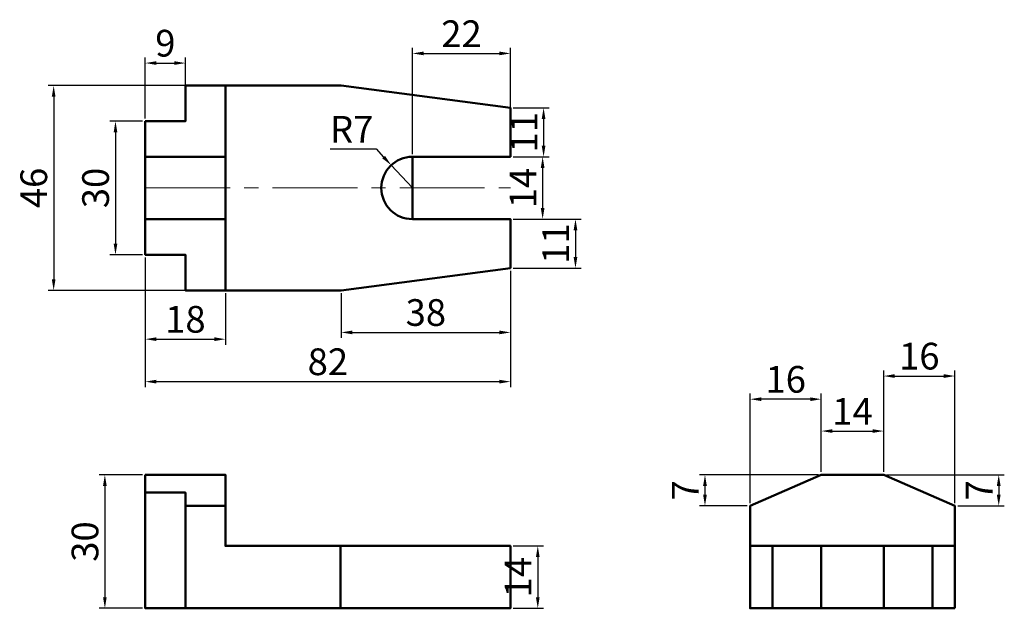
# Model space of a CAD drawing. Units: millimetres. Extents: x 44 to 265, y 73 to 205.
import ezdxf

# ---------------------------------------------------------------- set-up
doc = ezdxf.new("R2010")
doc.units = ezdxf.units.MM
doc.linetypes.add('CENTER2', pattern=[28.575, 19.05, -3.175, 3.175, -3.175])
for name, color, linetype, lineweight in [('M-CNTR', 1, 'CENTER2', 18), ('M-DIMS', 2, 'Continuous', 25), ('M-OUTL', 7, 'Continuous', 50)]:
    doc.layers.add(name, color=color, linetype=linetype, lineweight=lineweight)
doc.styles.get("Standard").update_dxf_attribs({"font": 'arial.ttf'})
doc.dimstyles.new('ISO-25', dxfattribs={"dimtxt": 6, "dimasz": 2.5, "dimexe": 1.25, "dimexo": 0.625, "dimtad": 1, "dimtoh": 1, "dimdec": 0, "dimtxsty": 'Standard', "dimcen": 2.5, "dimadec": 0, "dimazin": 0, "dimtfac": 1, "dimtdec": 0, "dimtmove": 0, "dimatfit": 3, "dimfxl": 1, "dimarcsym": 0})

# ---------------------------------------------------------------- blocks, each defined once
blk = doc.blocks.new('*D1')
at = {"layer": 'Defpoints', "color": 0, "transparency": 16777216}
for p in [(72.34, 152.49), (90.34, 144.49), (90.34, 133.53)]:
    blk.add_point(p, dxfattribs=at)
at = {"layer": 'M-DIMS', "color": 0, "lineweight": -2, "transparency": 16777216}
for p, q in [((72.34, 151.86), (72.34, 132.28)), ((90.34, 143.86), (90.34, 132.28)), ((74.84, 133.53), (87.84, 133.53))]:
    blk.add_line(p, q, dxfattribs=at)
at = {"layer": 'M-DIMS', "color": 0, "transparency": 16777216}
for points in [[(74.84, 133.95), (74.84, 133.11), (72.34, 133.53)], [(87.84, 133.95), (87.84, 133.11), (90.34, 133.53)]]:
    blk.add_solid(points, dxfattribs=at)
at = {"layer": 'M-DIMS', "color": 0, "transparency": 16777216, "insert": (81.34, 137.22), "char_height": 6, "attachment_point": 5}
blk.add_mtext('18', dxfattribs=at)
blk = doc.blocks.new('*D2')
at = {"layer": 'Defpoints', "color": 0, "transparency": 16777216}
for p in [(90.34, 190.49), (51.76, 144.49), (90.34, 144.49)]:
    blk.add_point(p, dxfattribs=at)
at = {"layer": 'M-DIMS', "color": 0, "lineweight": -2, "transparency": 16777216}
for p, q in [((89.71, 190.49), (50.51, 190.49)), ((51.76, 187.99), (51.76, 146.99)), ((89.71, 144.49), (50.51, 144.49))]:
    blk.add_line(p, q, dxfattribs=at)
at = {"layer": 'M-DIMS', "color": 0, "transparency": 16777216}
for points in [[(51.34, 187.99), (52.17, 187.99), (51.76, 190.49)], [(51.34, 146.99), (52.17, 146.99), (51.76, 144.49)]]:
    blk.add_solid(points, dxfattribs=at)
at = {"layer": 'M-DIMS', "color": 0, "transparency": 16777216, "insert": (48.07, 167.49), "char_height": 6, "attachment_point": 5, "rotation": 90}
blk.add_mtext('46', dxfattribs=at)
blk = doc.blocks.new('*D3')
at = {"layer": 'Defpoints', "color": 0, "transparency": 16777216}
for p in [(72.34, 182.49), (65.64, 152.49), (72.34, 152.49)]:
    blk.add_point(p, dxfattribs=at)
at = {"layer": 'M-DIMS', "color": 0, "lineweight": -2, "transparency": 16777216}
for p, q in [((71.71, 182.49), (64.39, 182.49)), ((65.64, 179.99), (65.64, 154.99)), ((71.71, 152.49), (64.39, 152.49))]:
    blk.add_line(p, q, dxfattribs=at)
at = {"layer": 'M-DIMS', "color": 0, "transparency": 16777216}
for points in [[(65.23, 179.99), (66.06, 179.99), (65.64, 182.49)], [(65.23, 154.99), (66.06, 154.99), (65.64, 152.49)]]:
    blk.add_solid(points, dxfattribs=at)
at = {"layer": 'M-DIMS', "color": 0, "transparency": 16777216, "insert": (61.95, 167.49), "char_height": 6, "attachment_point": 5, "rotation": 90}
blk.add_mtext('30', dxfattribs=at)
blk = doc.blocks.new('*D4')
at = {"layer": 'Defpoints', "color": 0, "transparency": 16777216}
for p in [(81.34, 195.54), (72.34, 182.49), (81.34, 182.49)]:
    blk.add_point(p, dxfattribs=at)
at = {"layer": 'M-DIMS', "color": 0, "lineweight": -2, "transparency": 16777216}
for p, q in [((72.34, 183.11), (72.34, 196.79)), ((81.34, 183.11), (81.34, 196.79)), ((74.84, 195.54), (78.84, 195.54))]:
    blk.add_line(p, q, dxfattribs=at)
at = {"layer": 'M-DIMS', "color": 0, "transparency": 16777216}
for points in [[(74.84, 195.96), (74.84, 195.13), (72.34, 195.54)], [(78.84, 195.96), (78.84, 195.13), (81.34, 195.54)]]:
    blk.add_solid(points, dxfattribs=at)
at = {"layer": 'M-DIMS', "color": 0, "transparency": 16777216, "insert": (76.84, 199.23), "char_height": 6, "attachment_point": 5}
blk.add_mtext('9', dxfattribs=at)
blk = doc.blocks.new('*D5')
at = {"layer": 'Defpoints', "color": 0, "transparency": 16777216}
for p in [(154.34, 197.71), (132.34, 174.49), (154.34, 174.49)]:
    blk.add_point(p, dxfattribs=at)
at = {"layer": 'M-DIMS', "color": 0, "lineweight": -2, "transparency": 16777216}
for p, q in [((132.34, 175.11), (132.34, 198.96)), ((134.84, 197.71), (151.84, 197.71)), ((154.34, 175.11), (154.34, 198.96))]:
    blk.add_line(p, q, dxfattribs=at)
at = {"layer": 'M-DIMS', "color": 0, "transparency": 16777216}
for points in [[(134.84, 198.13), (134.84, 197.3), (132.34, 197.71)], [(151.84, 198.13), (151.84, 197.3), (154.34, 197.71)]]:
    blk.add_solid(points, dxfattribs=at)
at = {"layer": 'M-DIMS', "color": 0, "transparency": 16777216, "insert": (143.34, 201.35), "char_height": 6, "attachment_point": 5}
blk.add_mtext('22', dxfattribs=at)
blk = doc.blocks.new('*D6')
at = {"layer": 'Defpoints', "color": 0, "transparency": 16777216}
for p in [(127.56, 172.61), (132.34, 167.49)]:
    blk.add_point(p, dxfattribs=at)
at = {"layer": 'M-DIMS', "color": 0, "lineweight": -2, "transparency": 16777216}
for p, q in [((113.85, 176.26), (124.15, 176.26)), ((124.15, 176.26), (125.86, 174.43)), ((132.34, 167.49), (127.56, 172.61))]:
    blk.add_line(p, q, dxfattribs=at)
at = {"layer": 'M-DIMS', "color": 0, "transparency": 16777216}
blk.add_solid([(126.16, 174.72), (125.55, 174.15), (127.56, 172.61)], dxfattribs=at)
at = {"layer": 'M-DIMS', "color": 0, "transparency": 16777216, "insert": (118.69, 179.89), "char_height": 6, "attachment_point": 5}
blk.add_mtext('R7', dxfattribs=at)
blk = doc.blocks.new('*D7')
at = {"layer": 'Defpoints', "color": 0, "transparency": 16777216}
for p in [(154.34, 185.49), (154.34, 174.49), (161.78, 174.49)]:
    blk.add_point(p, dxfattribs=at)
at = {"layer": 'M-DIMS', "color": 0, "lineweight": -2, "transparency": 16777216}
for p, q in [((154.96, 185.49), (163.03, 185.49)), ((161.78, 182.99), (161.78, 176.99)), ((154.96, 174.49), (163.03, 174.49))]:
    blk.add_line(p, q, dxfattribs=at)
at = {"layer": 'M-DIMS', "color": 0, "transparency": 16777216}
for points in [[(161.36, 182.99), (162.2, 182.99), (161.78, 185.49)], [(161.36, 176.99), (162.2, 176.99), (161.78, 174.49)]]:
    blk.add_solid(points, dxfattribs=at)
at = {"layer": 'M-DIMS', "color": 0, "transparency": 16777216, "insert": (158.14, 179.99), "char_height": 6, "attachment_point": 5, "rotation": 90}
blk.add_mtext('11', dxfattribs=at)
blk = doc.blocks.new('*D8')
at = {"layer": 'Defpoints', "color": 0, "transparency": 16777216}
for p in [(154.34, 174.49), (154.34, 160.49), (161.56, 160.49)]:
    blk.add_point(p, dxfattribs=at)
at = {"layer": 'M-DIMS', "color": 0, "lineweight": -2, "transparency": 16777216}
for p, q in [((154.96, 174.49), (162.81, 174.49)), ((161.56, 171.99), (161.56, 162.99)), ((154.96, 160.49), (162.81, 160.49))]:
    blk.add_line(p, q, dxfattribs=at)
at = {"layer": 'M-DIMS', "color": 0, "transparency": 16777216}
for points in [[(161.15, 171.99), (161.98, 171.99), (161.56, 174.49)], [(161.15, 162.99), (161.98, 162.99), (161.56, 160.49)]]:
    blk.add_solid(points, dxfattribs=at)
at = {"layer": 'M-DIMS', "color": 0, "transparency": 16777216, "insert": (157.93, 167.49), "char_height": 6, "attachment_point": 5, "rotation": 90}
blk.add_mtext('14', dxfattribs=at)
blk = doc.blocks.new('*D9')
at = {"layer": 'Defpoints', "color": 0, "transparency": 16777216}
for p in [(154.34, 160.49), (154.34, 149.49), (168.94, 149.49)]:
    blk.add_point(p, dxfattribs=at)
at = {"layer": 'M-DIMS', "color": 0, "lineweight": -2, "transparency": 16777216}
for p, q in [((154.96, 160.49), (170.19, 160.49)), ((168.94, 157.99), (168.94, 151.99)), ((154.96, 149.49), (170.19, 149.49))]:
    blk.add_line(p, q, dxfattribs=at)
at = {"layer": 'M-DIMS', "color": 0, "transparency": 16777216}
for points in [[(168.52, 157.99), (169.36, 157.99), (168.94, 160.49)], [(168.52, 151.99), (169.36, 151.99), (168.94, 149.49)]]:
    blk.add_solid(points, dxfattribs=at)
at = {"layer": 'M-DIMS', "color": 0, "transparency": 16777216, "insert": (165.3, 154.99), "char_height": 6, "attachment_point": 5, "rotation": 90}
blk.add_mtext('11', dxfattribs=at)
blk = doc.blocks.new('*D10')
at = {"layer": 'Defpoints', "color": 0, "transparency": 16777216}
for p in [(154.34, 149.49), (116.34, 144.49), (154.34, 135.05)]:
    blk.add_point(p, dxfattribs=at)
at = {"layer": 'M-DIMS', "color": 0, "lineweight": -2, "transparency": 16777216}
for p, q in [((154.34, 148.86), (154.34, 133.8)), ((116.34, 143.86), (116.34, 133.8)), ((118.84, 135.05), (151.84, 135.05))]:
    blk.add_line(p, q, dxfattribs=at)
at = {"layer": 'M-DIMS', "color": 0, "transparency": 16777216}
for points in [[(118.84, 135.46), (118.84, 134.63), (116.34, 135.05)], [(151.84, 135.46), (151.84, 134.63), (154.34, 135.05)]]:
    blk.add_solid(points, dxfattribs=at)
at = {"layer": 'M-DIMS', "color": 0, "transparency": 16777216, "insert": (135.34, 138.74), "char_height": 6, "attachment_point": 5}
blk.add_mtext('38', dxfattribs=at)
blk = doc.blocks.new('*D11')
at = {"layer": 'Defpoints', "color": 0, "transparency": 16777216}
for p in [(72.34, 152.49), (154.34, 149.49), (154.34, 123.99)]:
    blk.add_point(p, dxfattribs=at)
at = {"layer": 'M-DIMS', "color": 0, "lineweight": -2, "transparency": 16777216}
for p, q in [((72.34, 151.86), (72.34, 122.74)), ((154.34, 148.86), (154.34, 122.74)), ((74.84, 123.99), (151.84, 123.99))]:
    blk.add_line(p, q, dxfattribs=at)
at = {"layer": 'M-DIMS', "color": 0, "transparency": 16777216}
for points in [[(74.84, 124.41), (74.84, 123.57), (72.34, 123.99)], [(151.84, 124.41), (151.84, 123.57), (154.34, 123.99)]]:
    blk.add_solid(points, dxfattribs=at)
at = {"layer": 'M-DIMS', "color": 0, "transparency": 16777216, "insert": (113.34, 127.68), "char_height": 6, "attachment_point": 5}
blk.add_mtext('82', dxfattribs=at)
blk = doc.blocks.new('*D12')
at = {"layer": 'Defpoints', "color": 0, "transparency": 16777216}
for p in [(72.34, 103.08), (63.26, 73.08), (72.34, 73.08)]:
    blk.add_point(p, dxfattribs=at)
at = {"layer": 'M-DIMS', "color": 0, "lineweight": -2, "transparency": 16777216}
for p, q in [((71.71, 103.08), (62.01, 103.08)), ((63.26, 100.58), (63.26, 75.58)), ((71.71, 73.08), (62.01, 73.08))]:
    blk.add_line(p, q, dxfattribs=at)
at = {"layer": 'M-DIMS', "color": 0, "transparency": 16777216}
for points in [[(62.84, 100.58), (63.67, 100.58), (63.26, 103.08)], [(62.84, 75.58), (63.67, 75.58), (63.26, 73.08)]]:
    blk.add_solid(points, dxfattribs=at)
at = {"layer": 'M-DIMS', "color": 0, "transparency": 16777216, "insert": (59.57, 88.08), "char_height": 6, "attachment_point": 5, "rotation": 90}
blk.add_mtext('30', dxfattribs=at)
blk = doc.blocks.new('*D13')
at = {"layer": 'Defpoints', "color": 0, "transparency": 16777216}
for p in [(154.34, 87.08), (154.34, 73.08), (160.48, 73.08)]:
    blk.add_point(p, dxfattribs=at)
at = {"layer": 'M-DIMS', "color": 0, "lineweight": -2, "transparency": 16777216}
for p, q in [((154.96, 87.08), (161.73, 87.08)), ((160.48, 84.58), (160.48, 75.58)), ((154.96, 73.08), (161.73, 73.08))]:
    blk.add_line(p, q, dxfattribs=at)
at = {"layer": 'M-DIMS', "color": 0, "transparency": 16777216}
for points in [[(160.06, 84.58), (160.89, 84.58), (160.48, 87.08)], [(160.06, 75.58), (160.89, 75.58), (160.48, 73.08)]]:
    blk.add_solid(points, dxfattribs=at)
at = {"layer": 'M-DIMS', "color": 0, "transparency": 16777216, "insert": (156.84, 80.08), "char_height": 6, "attachment_point": 5, "rotation": 90}
blk.add_mtext('14', dxfattribs=at)
blk = doc.blocks.new('*D14')
at = {"layer": 'Defpoints', "color": 0, "transparency": 16777216}
for p in [(224.15, 103.08), (198.02, 96.08), (208.15, 96.08)]:
    blk.add_point(p, dxfattribs=at)
at = {"layer": 'M-DIMS', "color": 0, "lineweight": -2, "transparency": 16777216}
for p, q in [((223.52, 103.08), (196.77, 103.08)), ((198.02, 100.58), (198.02, 98.58)), ((207.52, 96.08), (196.77, 96.08))]:
    blk.add_line(p, q, dxfattribs=at)
at = {"layer": 'M-DIMS', "color": 0, "transparency": 16777216}
for points in [[(197.6, 100.58), (198.44, 100.58), (198.02, 103.08)], [(197.6, 98.58), (198.44, 98.58), (198.02, 96.08)]]:
    blk.add_solid(points, dxfattribs=at)
at = {"layer": 'M-DIMS', "color": 0, "transparency": 16777216, "insert": (194.39, 99.58), "char_height": 6, "attachment_point": 5, "rotation": 90}
blk.add_mtext('7', dxfattribs=at)
blk = doc.blocks.new('*D15')
at = {"layer": 'Defpoints', "color": 0, "transparency": 16777216}
for p in [(238.15, 103.08), (254.15, 96.08), (263.99, 96.08)]:
    blk.add_point(p, dxfattribs=at)
at = {"layer": 'M-DIMS', "color": 0, "lineweight": -2, "transparency": 16777216}
for p, q in [((238.77, 103.08), (265.24, 103.08)), ((263.99, 100.58), (263.99, 98.58)), ((254.77, 96.08), (265.24, 96.08))]:
    blk.add_line(p, q, dxfattribs=at)
at = {"layer": 'M-DIMS', "color": 0, "transparency": 16777216}
for points in [[(263.57, 100.58), (264.41, 100.58), (263.99, 103.08)], [(263.57, 98.58), (264.41, 98.58), (263.99, 96.08)]]:
    blk.add_solid(points, dxfattribs=at)
at = {"layer": 'M-DIMS', "color": 0, "transparency": 16777216, "insert": (260.37, 99.58), "char_height": 6, "attachment_point": 5, "rotation": 90}
blk.add_mtext('7', dxfattribs=at)
blk = doc.blocks.new('*D16')
at = {"layer": 'Defpoints', "color": 0, "transparency": 16777216}
for p in [(208.15, 120.05), (224.15, 103.08), (208.15, 96.08)]:
    blk.add_point(p, dxfattribs=at)
at = {"layer": 'M-DIMS', "color": 0, "lineweight": -2, "transparency": 16777216}
for p, q in [((208.15, 96.71), (208.15, 121.3)), ((221.65, 120.05), (210.65, 120.05)), ((224.15, 103.71), (224.15, 121.3))]:
    blk.add_line(p, q, dxfattribs=at)
at = {"layer": 'M-DIMS', "color": 0, "transparency": 16777216}
for points in [[(210.65, 120.46), (210.65, 119.63), (208.15, 120.05)], [(221.65, 120.46), (221.65, 119.63), (224.15, 120.05)]]:
    blk.add_solid(points, dxfattribs=at)
at = {"layer": 'M-DIMS', "color": 0, "transparency": 16777216, "insert": (216.15, 123.73), "char_height": 6, "attachment_point": 5}
blk.add_mtext('16', dxfattribs=at)
blk = doc.blocks.new('*D17')
at = {"layer": 'Defpoints', "color": 0, "transparency": 16777216}
for p in [(238.15, 112.89), (224.15, 103.08), (238.15, 103.08)]:
    blk.add_point(p, dxfattribs=at)
at = {"layer": 'M-DIMS', "color": 0, "lineweight": -2, "transparency": 16777216}
for p, q in [((224.15, 103.71), (224.15, 114.14)), ((226.65, 112.89), (235.65, 112.89)), ((238.15, 103.71), (238.15, 114.14))]:
    blk.add_line(p, q, dxfattribs=at)
at = {"layer": 'M-DIMS', "color": 0, "transparency": 16777216}
for points in [[(226.65, 113.31), (226.65, 112.47), (224.15, 112.89)], [(235.65, 113.31), (235.65, 112.47), (238.15, 112.89)]]:
    blk.add_solid(points, dxfattribs=at)
at = {"layer": 'M-DIMS', "color": 0, "transparency": 16777216, "insert": (231.15, 116.53), "char_height": 6, "attachment_point": 5}
blk.add_mtext('14', dxfattribs=at)
blk = doc.blocks.new('*D18')
at = {"layer": 'Defpoints', "color": 0, "transparency": 16777216}
for p in [(254.15, 125.25), (238.15, 103.08), (254.15, 96.08)]:
    blk.add_point(p, dxfattribs=at)
at = {"layer": 'M-DIMS', "color": 0, "lineweight": -2, "transparency": 16777216}
for p, q in [((238.15, 103.71), (238.15, 126.5)), ((254.15, 96.71), (254.15, 126.5)), ((240.65, 125.25), (251.65, 125.25))]:
    blk.add_line(p, q, dxfattribs=at)
at = {"layer": 'M-DIMS', "color": 0, "transparency": 16777216}
for points in [[(240.65, 125.67), (240.65, 124.83), (238.15, 125.25)], [(251.65, 125.67), (251.65, 124.83), (254.15, 125.25)]]:
    blk.add_solid(points, dxfattribs=at)
at = {"layer": 'M-DIMS', "color": 0, "transparency": 16777216, "insert": (246.15, 128.94), "char_height": 6, "attachment_point": 5}
blk.add_mtext('16', dxfattribs=at)

msp = doc.modelspace()

# ---------------------------------------------------------------- linework, layer by layer
at = {"layer": 'M-CNTR'}
msp.add_line((72.34, 167.49), (154.34, 167.49), dxfattribs=at)
at = {"layer": 'M-OUTL'}
for p, q in [((90.34, 190.49), (90.34, 144.49)), ((90.34, 174.49), (72.34, 174.49)), ((90.34, 160.49), (72.34, 160.49)), ((90.34, 96.08), (81.34, 96.08)), ((116.14, 87.08), (116.14, 73.08)), ((208.15, 87.08), (254.15, 87.08)), ((213.15, 73.08), (213.15, 87.08)), ((224.15, 73.08), (224.15, 87.08)), ((238.15, 73.08), (238.15, 87.08)), ((249.15, 73.08), (249.15, 87.08))]:
    msp.add_line(p, q, dxfattribs=at)
for points in [[(72.34, 182.49), (81.34, 182.49), (81.34, 190.49), (90.34, 190.49), (116.34, 190.49), (154.34, 185.49), (154.34, 174.49), (132.34, 174.49)], [(72.34, 99.08), (81.34, 99.08), (81.34, 73.08)]]:
    msp.add_lwpolyline(points, dxfattribs=at)
msp.add_lwpolyline([(72.34, 182.49), (72.34, 152.49), (81.34, 152.49), (81.34, 144.49), (90.34, 144.49), (116.34, 144.49), (154.34, 149.49), (154.34, 160.49), (132.34, 160.49, -1), (132.34, 174.49), (132.34, 160.49)], format="xyb", dxfattribs=at)
for points in [[(72.34, 103.08), (90.34, 103.08), (90.34, 87.08), (154.34, 87.08), (154.34, 73.08), (72.34, 73.08)], [(254.15, 73.08), (254.15, 96.08), (238.15, 103.08), (224.15, 103.08), (208.15, 96.08), (208.15, 73.08)]]:
    msp.add_lwpolyline(points, close=True, dxfattribs=at)

# ---------------------------------------------------------------- dimensions: what is measured, and where the dimension line sits
at = {"layer": 'M-DIMS'}
for base, p1, p2, picture, middle in [((154.34, 197.71), (132.34, 174.49), (154.34, 174.49), '*D5', (143.34, 201.35)), ((81.34, 195.54), (72.34, 182.49), (81.34, 182.49), '*D4', (76.84, 199.23)), ((90.34, 133.53), (72.34, 152.49), (90.34, 144.49), '*D1', (81.34, 137.22)), ((154.34, 123.99), (72.34, 152.49), (154.34, 149.49), '*D11', (113.34, 127.68)), ((154.34, 135.05), (116.34, 144.49), (154.34, 149.49), '*D10', (135.34, 138.74)), ((254.15, 125.25), (238.15, 103.08), (254.15, 96.08), '*D18', (246.15, 128.94)), ((208.15, 120.05), (224.15, 103.08), (208.15, 96.08), '*D16', (216.15, 123.73)), ((238.15, 112.89), (224.15, 103.08), (238.15, 103.08), '*D17', (231.15, 116.53))]:
    dim = msp.add_linear_dim(base=base, p1=p1, p2=p2, dimstyle='ISO-25', override={"dimclrd": 0, "dimclre": 0, "dimclrt": 0}, dxfattribs=at)
    dim.commit()
    dim.dimension.update_dxf_attribs({"geometry": picture, "text_midpoint": middle})
for base, p1, p2, picture, middle in [((51.76, 144.49), (90.34, 190.49), (90.34, 144.49), '*D2', (48.07, 167.49)), ((161.78, 174.49), (154.34, 185.49), (154.34, 174.49), '*D7', (158.14, 179.99)), ((65.64, 152.49), (72.34, 182.49), (72.34, 152.49), '*D3', (61.95, 167.49)), ((161.56, 160.49), (154.34, 174.49), (154.34, 160.49), '*D8', (157.93, 167.49)), ((168.94, 149.49), (154.34, 160.49), (154.34, 149.49), '*D9', (165.3, 154.99)), ((63.26, 73.08), (72.34, 103.08), (72.34, 73.08), '*D12', (59.57, 88.08)), ((198.02, 96.08), (224.15, 103.08), (208.15, 96.08), '*D14', (194.39, 99.58)), ((263.99, 96.08), (238.15, 103.08), (254.15, 96.08), '*D15', (260.37, 99.58)), ((160.48, 73.08), (154.34, 87.08), (154.34, 73.08), '*D13', (156.84, 80.08))]:
    dim = msp.add_linear_dim(base=base, p1=p1, p2=p2, angle=90, dimstyle='ISO-25', override={"dimclrd": 0, "dimclre": 0, "dimclrt": 0}, dxfattribs=at)
    dim.commit()
    dim.dimension.update_dxf_attribs({"geometry": picture, "text_midpoint": middle})
dim = msp.add_radius_dim(center=(132.34, 167.49), mpoint=(127.56, 172.61), dimstyle='ISO-25', override={"dimclrd": 0, "dimclre": 0, "dimclrt": 0}, dxfattribs=at)
dim.commit()
dim.dimension.update_dxf_attribs({"geometry": '*D6', "text_midpoint": (118.69, 179.89)})

doc.saveas('drawing.dxf')
